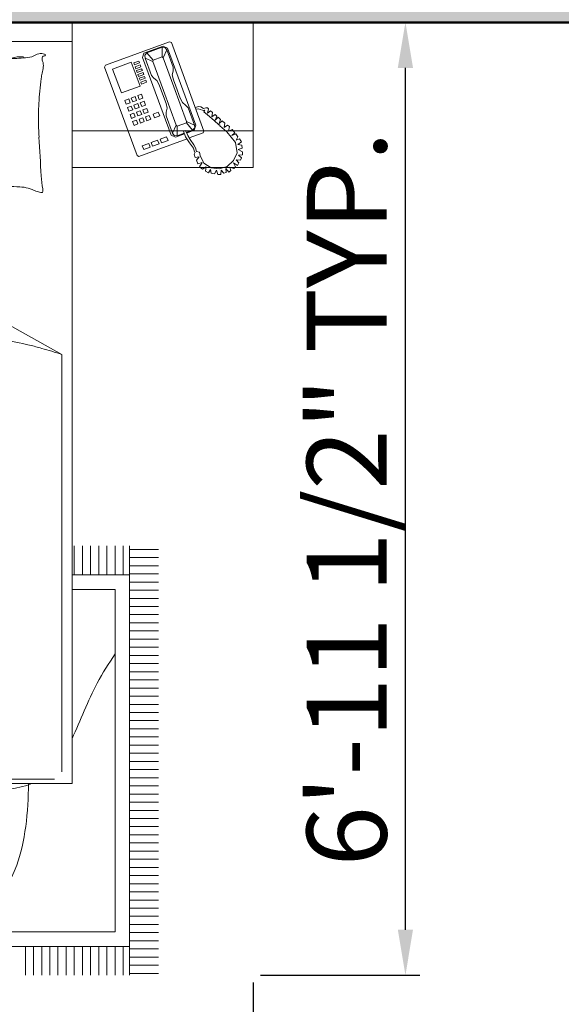
# Model space of a CAD drawing. Units: inches. Extents: x -7 to 1228, y -146 to 1091.
# Tile 12 of 88: x 153 to 200, y 401 to 487. Entities that reach past the tile are written whole.
import ezdxf

# ---------------------------------------------------------------- set-up
doc = ezdxf.new("R2010")
doc.units = ezdxf.units.IN
for name, color, linetype, lineweight in [('A-ANNO-DIMS', 2, 'Continuous', 18), ('A-FURN', 8, 'Continuous', 18), ('A-WALL', 7, 'Continuous', 50), ('A-WALL-PATT', 251, 'Continuous', 13)]:
    doc.layers.add(name, color=color, linetype=linetype, lineweight=lineweight)
doc.styles.add('DIM_FONT', font='SIMPLEX.shx', dxfattribs={"width": 0.8})
doc.styles.get("Standard").update_dxf_attribs({"font": 'arial.ttf'})
doc.dimstyles.new('ISO-25', dxfattribs={"dimtxt": 7, "dimasz": 4, "dimexe": 1.25, "dimexo": 0.625, "dimtad": 1, "dimdec": 1, "dimlunit": 3, "dimtxsty": 'Standard', "dimcen": 2.5, "dimadec": 0, "dimazin": 0, "dimtfac": 1, "dimtdec": 1, "dimtmove": 1, "dimatfit": 3, "dimfxl": 1, "dimarcsym": 0})

# ---------------------------------------------------------------- blocks, each defined once
blk = doc.blocks.new('A$C4F634EDD')
for p, q in [((0.5, 2.6295), (2.3, 2.6295)), ((2.3, 2.6295), (2.3, 0.5295)), ((2.3, 2.6295), (2.8, 2.6295)), ((2.3, 2.2295), (2.3, 2.6295)), ((2.8, 2.6295), (2.8, 2.2295)), ((0.5, 2.5771), (2.3, 2.5771)), ((2.392, 2.5115), (2.5692, 2.5765)), ((2.4985, 2.5445), (2.5516, 2.564)), ((2.5062, 2.5454), (2.5487, 2.561)), ((2.5483, 2.5347), (2.5487, 2.561)), ((2.5487, 2.561), (2.5571, 2.56)), ((2.5516, 2.564), (2.5637, 2.5584)), ((2.5571, 2.56), (2.5615, 2.5536)), ((2.5637, 2.5584), (2.6418, 2.3458)), ((2.5692, 2.5765), (2.574, 2.5743)), ((2.574, 2.5743), (2.6638, 2.3298)), ((2.4946, 2.5331), (2.4985, 2.5445)), ((2.5734, 2.3187), (2.4946, 2.5331)), ((2.5062, 2.5454), (2.5004, 2.5392)), ((2.5004, 2.5392), (2.5013, 2.5315)), ((2.5013, 2.5315), (2.5188, 2.4836)), ((2.5013, 2.5315), (2.5231, 2.5214)), ((2.5235, 2.5256), (2.5062, 2.5454)), ((2.5483, 2.5347), (2.5235, 2.5256)), ((2.5514, 2.5318), (2.5483, 2.5347)), ((2.5615, 2.5536), (2.5514, 2.5318)), ((2.5807, 2.4521), (2.5514, 2.5318)), ((2.5615, 2.5536), (2.5791, 2.5058)), ((2.3898, 2.5066), (2.392, 2.5115)), ((2.4795, 2.2621), (2.3898, 2.5066)), ((2.412, 2.5007), (2.4634, 2.5196)), ((2.4361, 2.4352), (2.412, 2.5007)), ((2.4634, 2.5196), (2.4875, 2.454)), ((2.4842, 2.5232), (2.47, 2.518)), ((2.47, 2.518), (2.472, 2.5127)), ((2.472, 2.5127), (2.4862, 2.5179)), ((2.4881, 2.5126), (2.4739, 2.5074)), ((2.4739, 2.5074), (2.4759, 2.502)), ((2.4759, 2.502), (2.4901, 2.5073)), ((2.492, 2.5019), (2.4778, 2.4967)), ((2.4862, 2.5179), (2.4842, 2.5232)), ((2.4901, 2.5073), (2.4881, 2.5126)), ((2.494, 2.4966), (2.492, 2.5019)), ((2.5231, 2.5214), (2.5235, 2.5256)), ((2.5523, 2.4417), (2.5231, 2.5214)), ((2.5791, 2.5058), (2.5788, 2.4956)), ((2.4778, 2.4967), (2.4798, 2.4914)), ((2.4798, 2.4914), (2.494, 2.4966)), ((2.4959, 2.4913), (2.4817, 2.4861)), ((2.4817, 2.4861), (2.4837, 2.4808)), ((2.4837, 2.4808), (2.4979, 2.486)), ((2.4998, 2.4807), (2.4856, 2.4755)), ((2.4856, 2.4755), (2.4876, 2.4702)), ((2.4876, 2.4702), (2.5018, 2.4754)), ((2.4979, 2.486), (2.4959, 2.4913)), ((2.5018, 2.4754), (2.4998, 2.4807)), ((2.5188, 2.4836), (2.5256, 2.4761)), ((2.5256, 2.4761), (2.5342, 2.4692)), ((2.5788, 2.4956), (2.5767, 2.4848)), ((2.5767, 2.4848), (2.5795, 2.4717)), ((2.4875, 2.454), (2.4361, 2.4352)), ((2.5037, 2.47), (2.4895, 2.4648)), ((2.4895, 2.4648), (2.4915, 2.4595)), ((2.4915, 2.4595), (2.5057, 2.4647)), ((2.5057, 2.4647), (2.5037, 2.47)), ((2.5342, 2.4692), (2.5405, 2.4574)), ((2.5405, 2.4574), (2.547, 2.4397)), ((2.5795, 2.4717), (2.586, 2.454)), ((2.5807, 2.4521), (2.6158, 2.3564)), ((2.5984, 2.4204), (2.586, 2.454)), ((2.4457, 2.4146), (2.4563, 2.4185)), ((2.4563, 2.4185), (2.4602, 2.4078)), ((2.4634, 2.4211), (2.474, 2.425)), ((2.4673, 2.4104), (2.4634, 2.4211)), ((2.474, 2.425), (2.4779, 2.4143)), ((2.4811, 2.4276), (2.4917, 2.4315)), ((2.485, 2.4169), (2.4811, 2.4276)), ((2.4956, 2.4208), (2.485, 2.4169)), ((2.4917, 2.4315), (2.4956, 2.4208)), ((2.5594, 2.4061), (2.547, 2.4397)), ((2.5523, 2.4417), (2.5875, 2.346)), ((2.6047, 2.4086), (2.5984, 2.4204)), ((2.4496, 2.4039), (2.4457, 2.4146)), ((2.4602, 2.4078), (2.4496, 2.4039)), ((2.4528, 2.3951), (2.4635, 2.399)), ((2.4567, 2.3844), (2.4528, 2.3951)), ((2.4635, 2.399), (2.4674, 2.3883)), ((2.4779, 2.4143), (2.4673, 2.4104)), ((2.4706, 2.4016), (2.4812, 2.4055)), ((2.4745, 2.3909), (2.4706, 2.4016)), ((2.4851, 2.3949), (2.4745, 2.3909)), ((2.4812, 2.4055), (2.4851, 2.3949)), ((2.4883, 2.4081), (2.4989, 2.412)), ((2.4922, 2.3975), (2.4883, 2.4081)), ((2.5028, 2.4014), (2.4922, 2.3975)), ((2.4954, 2.3886), (2.5061, 2.3925)), ((2.4989, 2.412), (2.5028, 2.4014)), ((2.5061, 2.3925), (2.51, 2.3819)), ((2.5622, 2.393), (2.5594, 2.4061)), ((2.5601, 2.3822), (2.5622, 2.393)), ((2.6133, 2.4017), (2.6047, 2.4086)), ((2.6201, 2.3941), (2.6133, 2.4017)), ((2.6376, 2.3463), (2.6201, 2.3941)), ((2.6499, 2.3979), (2.6397, 2.3953)), ((2.6551, 2.397), (2.6499, 2.3979)), ((2.6627, 2.392), (2.6551, 2.397)), ((2.6692, 2.394), (2.6627, 2.392)), ((2.6736, 2.3944), (2.6692, 2.394)), ((2.6765, 2.391), (2.6736, 2.3944)), ((2.4674, 2.3883), (2.4567, 2.3844)), ((2.46, 2.3756), (2.4706, 2.3795)), ((2.4639, 2.365), (2.46, 2.3756)), ((2.4745, 2.3689), (2.4639, 2.365)), ((2.4706, 2.3795), (2.4745, 2.3689)), ((2.4777, 2.3821), (2.4883, 2.386)), ((2.4816, 2.3715), (2.4777, 2.3821)), ((2.4922, 2.3754), (2.4816, 2.3715)), ((2.4849, 2.3626), (2.4955, 2.3665)), ((2.4883, 2.386), (2.4922, 2.3754)), ((2.4993, 2.378), (2.4954, 2.3886)), ((2.4955, 2.3665), (2.4994, 2.3559)), ((2.51, 2.3819), (2.4993, 2.378)), ((2.5026, 2.3691), (2.5132, 2.373)), ((2.5065, 2.3585), (2.5026, 2.3691)), ((2.5132, 2.373), (2.5171, 2.3624)), ((2.5238, 2.3769), (2.538, 2.3821)), ((2.5277, 2.3663), (2.5238, 2.3769)), ((2.5419, 2.3715), (2.5277, 2.3663)), ((2.538, 2.3821), (2.5419, 2.3715)), ((2.5598, 2.372), (2.5601, 2.3822)), ((2.5774, 2.3242), (2.5598, 2.372)), ((2.6417, 2.39), (2.6488, 2.391)), ((2.6488, 2.391), (2.6538, 2.3895)), ((2.6538, 2.3895), (2.6596, 2.388)), ((2.6596, 2.388), (2.6626, 2.3867)), ((2.6626, 2.3867), (2.6662, 2.388)), ((2.6662, 2.388), (2.6632, 2.3828)), ((2.6632, 2.3828), (2.6736, 2.3744)), ((2.6736, 2.3744), (2.6922, 2.3593)), ((2.6742, 2.3795), (2.6765, 2.391)), ((2.6824, 2.3858), (2.6742, 2.3795)), ((2.6873, 2.3815), (2.6824, 2.3858)), ((2.6853, 2.369), (2.6873, 2.3815)), ((2.6946, 2.376), (2.6853, 2.369)), ((2.6995, 2.3713), (2.6946, 2.376)), ((2.695, 2.3603), (2.6995, 2.3713)), ((2.7031, 2.3682), (2.695, 2.3603)), ((2.7096, 2.3616), (2.7031, 2.3682)), ((2.4672, 2.3561), (2.4778, 2.36)), ((2.4711, 2.3455), (2.4672, 2.3561)), ((2.4817, 2.3494), (2.4711, 2.3455)), ((2.4778, 2.36), (2.4817, 2.3494)), ((2.4888, 2.352), (2.4849, 2.3626)), ((2.4994, 2.3559), (2.4888, 2.352)), ((2.5171, 2.3624), (2.5065, 2.3585)), ((2.5774, 2.3242), (2.5875, 2.346)), ((2.5875, 2.346), (2.5905, 2.3431)), ((2.5905, 2.3431), (2.5901, 2.3168)), ((2.6154, 2.3522), (2.5905, 2.3431)), ((2.6158, 2.3564), (2.6154, 2.3522)), ((2.6154, 2.3522), (2.6327, 2.3324)), ((2.6376, 2.3463), (2.6158, 2.3564)), ((2.6327, 2.3324), (2.6385, 2.3386)), ((2.6418, 2.3458), (2.6369, 2.332)), ((2.6385, 2.3386), (2.6376, 2.3463)), ((2.6922, 2.3593), (2.7051, 2.3473)), ((2.7051, 2.3473), (2.7079, 2.3475)), ((2.7062, 2.351), (2.7096, 2.3616)), ((2.7147, 2.3578), (2.7062, 2.351)), ((2.7079, 2.3475), (2.7079, 2.3443)), ((2.7079, 2.3443), (2.727, 2.3277)), ((2.7214, 2.3517), (2.7147, 2.3578)), ((2.7196, 2.34), (2.7214, 2.3517)), ((2.7286, 2.3466), (2.7196, 2.34)), ((2.7346, 2.3423), (2.7286, 2.3466)), ((2.732, 2.3295), (2.7346, 2.3423)), ((2.8, 2.3301), (2.3, 2.3301)), ((2.561, 2.3141), (2.5433, 2.3076)), ((2.5649, 2.3035), (2.561, 2.3141)), ((2.5855, 2.3131), (2.5734, 2.3187)), ((2.5818, 2.3178), (2.5774, 2.3242)), ((2.5901, 2.3168), (2.5818, 2.3178)), ((2.6104, 2.3222), (2.5855, 2.3131)), ((2.5901, 2.3168), (2.6097, 2.324)), ((2.613, 2.3312), (2.6077, 2.3293)), ((2.6077, 2.3293), (2.6135, 2.3141)), ((2.6192, 2.3174), (2.613, 2.3312)), ((2.6135, 2.3141), (2.6244, 2.2977)), ((2.6153, 2.3261), (2.6327, 2.3324)), ((2.6369, 2.332), (2.6161, 2.3243)), ((2.626, 2.3069), (2.6192, 2.3174)), ((2.6616, 2.3249), (2.6234, 2.3109)), ((2.6638, 2.3298), (2.6616, 2.3249)), ((2.727, 2.3277), (2.7512, 2.2983)), ((2.7423, 2.3345), (2.732, 2.3295)), ((2.7406, 2.3172), (2.7495, 2.325)), ((2.7519, 2.3218), (2.7406, 2.3172)), ((2.7495, 2.325), (2.7423, 2.3345)), ((2.7575, 2.3144), (2.7519, 2.3218)), ((2.7526, 2.3045), (2.7575, 2.3144)), ((2.6172, 2.3086), (2.4844, 2.2599)), ((2.5114, 2.2959), (2.4936, 2.2894)), ((2.4936, 2.2894), (2.4976, 2.2788)), ((2.4976, 2.2788), (2.5153, 2.2853)), ((2.5153, 2.2853), (2.5114, 2.2959)), ((2.5362, 2.305), (2.5185, 2.2985)), ((2.5185, 2.2985), (2.5224, 2.2879)), ((2.5224, 2.2879), (2.5401, 2.2944)), ((2.5401, 2.2944), (2.5362, 2.305)), ((2.5433, 2.3076), (2.5472, 2.297)), ((2.5472, 2.297), (2.5649, 2.3035)), ((2.6244, 2.2977), (2.6349, 2.2825)), ((2.6365, 2.2916), (2.626, 2.3069)), ((2.6349, 2.2825), (2.638, 2.273)), ((2.6407, 2.2834), (2.6365, 2.2916)), ((2.6438, 2.2739), (2.6407, 2.2834)), ((2.7512, 2.2983), (2.756, 2.2695)), ((2.7622, 2.308), (2.7526, 2.3045)), ((2.7574, 2.2924), (2.7673, 2.2997)), ((2.7687, 2.2905), (2.7574, 2.2924)), ((2.7587, 2.279), (2.7699, 2.2828)), ((2.7673, 2.2997), (2.7622, 2.308)), ((2.7699, 2.2828), (2.7687, 2.2905)), ((2.4844, 2.2599), (2.4795, 2.2621)), ((2.6399, 2.2712), (2.6374, 2.2659)), ((2.6374, 2.2659), (2.6398, 2.257)), ((2.638, 2.273), (2.6399, 2.2712)), ((2.6398, 2.257), (2.6509, 2.259)), ((2.6509, 2.259), (2.6431, 2.2492)), ((2.6519, 2.2716), (2.6438, 2.2739)), ((2.6535, 2.2628), (2.6519, 2.2716)), ((2.6636, 2.2409), (2.6535, 2.2628)), ((2.756, 2.2695), (2.7459, 2.2483)), ((2.7708, 2.2725), (2.7587, 2.279)), ((2.759, 2.2637), (2.7706, 2.2643)), ((2.7676, 2.2559), (2.759, 2.2637)), ((2.7645, 2.2498), (2.7676, 2.2559)), ((2.7706, 2.2643), (2.7708, 2.2725)), ((2.8, 2.2295), (2.3, 2.2295)), ((2.6431, 2.2492), (2.6473, 2.2398)), ((2.6473, 2.2398), (2.6592, 2.2429)), ((2.6592, 2.2429), (2.6521, 2.2314)), ((2.6521, 2.2314), (2.6598, 2.2248)), ((2.6598, 2.2248), (2.6697, 2.2309)), ((2.6836, 2.2287), (2.6636, 2.2409)), ((2.6697, 2.2309), (2.6684, 2.219)), ((2.7063, 2.2256), (2.6836, 2.2287)), ((2.7284, 2.2317), (2.7063, 2.2256)), ((2.7459, 2.2483), (2.7284, 2.2317)), ((2.7386, 2.2208), (2.7354, 2.2306)), ((2.7354, 2.2306), (2.7462, 2.2264)), ((2.7509, 2.2314), (2.7459, 2.2418)), ((2.7459, 2.2418), (2.7568, 2.2352)), ((2.7462, 2.2264), (2.7509, 2.2314)), ((2.7529, 2.2505), (2.7645, 2.2498)), ((2.7607, 2.2424), (2.7529, 2.2505)), ((2.7568, 2.2352), (2.7607, 2.2424)), ((2.6684, 2.219), (2.6761, 2.2145)), ((2.6761, 2.2145), (2.6821, 2.2237)), ((2.6821, 2.2237), (2.6843, 2.2135)), ((2.6843, 2.2135), (2.6927, 2.2117)), ((2.6927, 2.2117), (2.6986, 2.222)), ((2.6986, 2.222), (2.7019, 2.2098)), ((2.7019, 2.2098), (2.7102, 2.2104)), ((2.7102, 2.2104), (2.7113, 2.2218)), ((2.7113, 2.2218), (2.7192, 2.2137)), ((2.7192, 2.2137), (2.7255, 2.2152)), ((2.7255, 2.2152), (2.7242, 2.2265)), ((2.7242, 2.2265), (2.7324, 2.2165)), ((2.7324, 2.2165), (2.7386, 2.2208)), ((1.5035, 2.141), (2.2716, 1.7136)), ((2.2716, 0.5617), (2.2716, 1.7136)), ((2.3061, 1.1052), (2.3061, 1.1852)), ((2.3286, 1.1052), (2.3286, 1.1852)), ((2.3511, 1.1052), (2.3511, 1.1852)), ((2.3736, 1.1052), (2.3736, 1.1852)), ((2.3961, 1.1052), (2.3961, 1.1852)), ((2.4186, 1.1052), (2.4186, 1.1852)), ((2.4411, 1.1052), (2.4411, 1.1852)), ((2.4588, 1.1852), (2.4588, 0)), ((2.4588, 1.1753), (2.5388, 1.1753)), ((2.4588, 1.1528), (2.5388, 1.1528)), ((2.4588, 1.1303), (2.5388, 1.1303)), ((2.3, 1.1052), (2.4588, 1.1052)), ((2.4588, 1.1078), (2.5388, 1.1078)), ((2.3, 1.0652), (2.4188, 1.0652)), ((2.4188, 1.0652), (2.4188, 0.12)), ((2.4588, 1.0853), (2.5388, 1.0853)), ((2.4588, 1.0628), (2.5388, 1.0628)), ((2.4588, 1.0403), (2.5388, 1.0403)), ((2.4588, 1.0178), (2.5388, 1.0178)), ((2.4588, 0.9953), (2.5388, 0.9953)), ((2.4588, 0.9728), (2.5388, 0.9728)), ((2.4588, 0.9503), (2.5388, 0.9503)), ((2.4588, 0.9278), (2.5388, 0.9278)), ((2.4588, 0.9053), (2.5388, 0.9053)), ((2.4588, 0.8828), (2.5388, 0.8828)), ((2.4588, 0.8603), (2.5388, 0.8603)), ((2.4588, 0.8378), (2.5388, 0.8378)), ((2.4588, 0.8153), (2.5388, 0.8153)), ((2.4588, 0.7928), (2.5388, 0.7928)), ((2.4588, 0.7703), (2.5388, 0.7703)), ((2.4588, 0.7478), (2.5388, 0.7478)), ((2.4588, 0.7253), (2.5388, 0.7253)), ((2.4588, 0.7028), (2.5388, 0.7028)), ((2.4588, 0.6803), (2.5388, 0.6803)), ((2.4588, 0.6578), (2.5388, 0.6578)), ((2.4588, 0.6353), (2.5388, 0.6353)), ((2.4588, 0.6128), (2.5388, 0.6128)), ((2.4588, 0.5903), (2.5388, 0.5903)), ((2.4588, 0.5678), (2.5388, 0.5678)), ((2.4588, 0.5453), (2.5388, 0.5453)), ((2.3, 0.5295), (0.5, 0.5295)), ((0.5458, 0.5417), (2.2516, 0.5417)), ((2.4588, 0.5228), (2.5388, 0.5228)), ((2.4588, 0.5003), (2.5388, 0.5003)), ((2.4588, 0.4778), (2.5388, 0.4778)), ((2.4588, 0.4553), (2.5388, 0.4553)), ((2.4588, 0.4328), (2.5388, 0.4328)), ((2.4588, 0.4103), (2.5388, 0.4103)), ((2.4588, 0.3878), (2.5388, 0.3878)), ((2.4588, 0.3653), (2.5388, 0.3653)), ((2.4588, 0.3428), (2.5388, 0.3428)), ((2.4588, 0.3203), (2.5388, 0.3203)), ((2.4588, 0.2978), (2.5388, 0.2978)), ((2.4588, 0.2753), (2.5388, 0.2753)), ((2.4588, 0.2528), (2.5388, 0.2528)), ((2.4588, 0.2303), (2.5388, 0.2303)), ((2.4588, 0.2078), (2.5388, 0.2078)), ((2.4588, 0.1853), (2.5388, 0.1853)), ((2.4588, 0.1628), (2.5388, 0.1628)), ((2.4588, 0.1403), (2.5388, 0.1403)), ((2.4188, 0.12), (0.3786, 0.12)), ((2.4588, 0.1178), (2.5388, 0.1178)), ((2.4588, 0.0953), (2.5388, 0.0953)), ((2.4588, 0.08), (0.3386, 0.08)), ((2.1711, 0), (2.1711, 0.08)), ((2.1936, 0), (2.1936, 0.08)), ((2.2161, 0), (2.2161, 0.08)), ((2.2386, 0), (2.2386, 0.08)), ((2.2611, 0), (2.2611, 0.08)), ((2.2836, 0), (2.2836, 0.08)), ((2.3061, 0), (2.3061, 0.08)), ((2.3286, 0), (2.3286, 0.08)), ((2.3511, 0), (2.3511, 0.08)), ((2.3736, 0), (2.3736, 0.08)), ((2.3961, 0), (2.3961, 0.08)), ((2.4186, 0), (2.4186, 0.08)), ((2.4411, 0), (2.4411, 0.08)), ((2.4588, 0.0728), (2.5388, 0.0728)), ((2.4588, 0.0503), (2.5388, 0.0503)), ((2.4588, 0.0278), (2.5388, 0.0278)), ((2.4588, 0.0053), (2.5388, 0.0053))]:
    blk.add_line(p, q)
for centre, radius, start, end in [((2.1021, 3.3501), 0.8208, 271.9079, 275.2592), ((2.1588, 2.4357), 0.0992, 85.7841, 105.9352), ((2.1724, 2.5864), 0.0539, 275.2592, 300.6513), ((2.2146, 2.5152), 0.0289, 85.6975, 120.6513), ((2.2149, 2.519), 0.0251, 68.2117, 85.6975), ((2.2331, 2.5288), 0.0156, 158.0096, 201.421), ((2.2226, 2.533), 0.00428, 78.1069, 158.0096), ((2.224, 2.5395), 0.00232, 258.1069, 19.564), ((2.2229, 2.5391), 0.00342, 19.564, 68.2117), ((1.977, 2.5413), 0.246, 347.8905, 351.8665), ((2.1881, 2.5111), 0.0328, 351.8665, 21.421), ((3.1198, 2.3525), 0.9131, 172.3191, 176.6313), ((2.4114, 2.448), 0.1983, 167.8905, 172.3191), ((2.8858, 2.3663), 0.6787, 176.6313, 181.6331), ((3.5721, 2.3859), 1.3652, 181.6331, 183.055), ((15.8249, 3.0398), 13.6356, 183.05496, 183.50486), ((2.5355, 2.2258), 0.3212, 183.5049, 189.9984), ((2.0833, 1.0141), 1.164, 86.426, 89.7135), ((2.1467, 2.0302), 0.1459, 77.131, 86.426), ((2.1691, 2.1283), 0.0453, 62.7159, 77.131), ((2.2251, 2.2367), 0.0767, 242.7159, 253.7788), ((2.2281, 2.247), 0.0875, 253.7788, 262.8796), ((2.2174, 2.1615), 0.00132, 262.8796, 343.3022), ((2.2001, 2.1667), 0.0193, 343.3022, 9.9984), ((1.2737, -2.2227), 4.0646, 77.0745, 79.2724), ((2.0359, 1.0981), 0.6574, 74.0648, 77.0745), ((1.7125, -0.0344), 1.8351, 72.2636, 74.0648)]:
    blk.add_arc(centre, radius, start, end)
for points, knots in [([(2.3, 0.6535), (2.3236, 0.7026), (2.3554, 0.7914), (2.4015, 0.8608), (2.4188, 0.8868)], [1893.525221, 1893.525221, 1893.525221, 1893.525221, 2051.902476, 2146.74457, 2146.74457, 2146.74457, 2146.74457]), ([(2.1796, 0.5295), (2.1798, 0.4519), (2.1548, 0.2369), (2.0487, 0.164), (1.9846, 0.12)], [2202.034493, 2202.034493, 2202.034493, 2202.034493, 2357.807635, 2594.446174, 2594.446174, 2594.446174, 2594.446174])]:
    blk.add_open_spline(points, degree=3, knots=knots)
blk.add_open_spline([(1.9003, 0.5295), (2.0065, 0.514), (2.1132, 0.4978), (2.1894, 0.5295)], degree=3)
at = {"style": 'DIM_FONT', "width": 0.8, "flags": 9}
for tag, p in [('YSIZE', (0.5, 2.6295)), ('XSIZE', (0.5, 2.6295)), ('XSIZE', (2.2985, 2.6295)), ('YSIZE', (2.2985, 2.6295))]:
    blk.add_attdef(tag, p, '', height=0.0005, dxfattribs=at)
blk = doc.blocks.new('*D24')
at = {"layer": 'A-ANNO-DIMS', "color": 0, "lineweight": -2, "transparency": 16777216}
for p, q in [((84.435, 402.798), (84.435, 388.824)), ((173.431, 402.798), (173.431, 388.824)), ((88.435, 390.074), (169.431, 390.074))]:
    blk.add_line(p, q, dxfattribs=at)
at = {"layer": 'A-ANNO-DIMS', "color": 0, "transparency": 16777216}
for points in [[(88.435, 390.741), (88.435, 389.407), (84.435, 390.074)], [(169.431, 390.741), (169.431, 389.407), (173.431, 390.074)]]:
    blk.add_solid(points, dxfattribs=at)
at = {"layer": 'Defpoints', "color": 0, "transparency": 16777216}
for p in [(84.435, 403.423), (173.431, 403.423), (173.431, 390.074)]:
    blk.add_point(p, dxfattribs=at)
at = {"layer": 'A-ANNO-DIMS', "color": 0, "transparency": 16777216, "insert": (128.933, 394.259), "char_height": 7, "attachment_point": 5}
blk.add_mtext('BED 7\'-5" TYP.', dxfattribs=at)
blk = doc.blocks.new('*D25')
at = {"layer": 'A-ANNO-DIMS', "color": 0, "lineweight": -2, "transparency": 16777216}
for p, q in [((174.056, 487.016), (188.031, 487.016)), ((186.781, 407.423), (186.781, 483.016)), ((174.056, 403.423), (188.031, 403.423))]:
    blk.add_line(p, q, dxfattribs=at)
at = {"layer": 'A-ANNO-DIMS', "color": 0, "transparency": 16777216}
for points in [[(186.114, 483.016), (187.447, 483.016), (186.781, 487.016)], [(186.114, 407.423), (187.447, 407.423), (186.781, 403.423)]]:
    blk.add_solid(points, dxfattribs=at)
at = {"layer": 'Defpoints', "color": 0, "transparency": 16777216}
for p in [(173.431, 487.016), (186.781, 487.016), (173.431, 403.423)]:
    blk.add_point(p, dxfattribs=at)
at = {"layer": 'A-ANNO-DIMS', "color": 0, "transparency": 16777216, "insert": (182.536, 445.22), "char_height": 7, "attachment_point": 5, "rotation": 90}
blk.add_mtext('6\'-11 1/2" TYP.', dxfattribs=at)

msp = doc.modelspace()

# ---------------------------------------------------------------- hatches: boundary and pattern name
at = {"layer": 'A-WALL-PATT'}
h = msp.add_hatch(color=256, dxfattribs=at)
h.dxf.hatch_style = 1
h.paths.add_polyline_path([(69, 568), (60, 568), (60, 493), (63.289, 493), (69, 493)])
h.paths.add_polyline_path([(69, 662.405), (60, 662.405), (60, 586), (69, 586)], flags=17)
h.paths.add_polyline_path([(69, 723), (184, 723), (184, 734), (179, 734), (179, 728), (69, 728), (69, 741.623), (60, 741.623), (60, 698.405), (69, 698.405)], flags=17)
h.paths.add_polyline_path([(69, 782), (231, 782), (231, 728), (231, 723), (231, 586), (236, 586), (236, 787), (69, 787), (69, 800.126), (60, 800.126), (60, 765.623), (69, 765.623)])
h.paths.add_polyline_path([(184, 842), (189, 842), (189, 848), (173, 848), (173, 842), (179, 842), (179, 787), (184, 787)])
h.paths.add_polyline_path([(118.22, 69), (69, 69), (69, 60), (118.22, 60)])
h.paths.add_polyline_path([(227, 69), (154.22, 69), (154.22, 60), (227, 60)])
h.paths.add_polyline_path([(236, 60), (232.711, 60), (227, 60), (227, 36), (236, 36)])
h.paths.add_polyline_path([(389, 60), (380, 60), (380, 36), (389, 36)])
h.paths.add_polyline_path([(384, 181), (380, 181), (380, 115), (380, 78), (384, 78)])
h.paths.add_polyline_path([(380, 115), (334.547, 115), (334.547, 109), (380, 109)])
h.paths.add_polyline_path([(274.547, 115), (236, 115), (236, 201), (232.711, 201), (231, 201), (231, 78), (236, 78), (236, 109), (274.547, 109)])
h.paths.add_polyline_path([(69, 123), (60, 123), (60, 78), (69, 78)])
h.paths.add_polyline_path([(69, 201), (60, 201), (60, 159), (69, 159)])
h.paths.add_polyline_path([(143, 219), (69, 219), (69, 213), (143, 213)], flags=17)
h.paths.add_polyline_path([(189, 219), (184, 219), (184, 274), (231, 274), (231, 219), (236, 219), (236, 279), (184, 279), (184, 297), (179, 297), (179, 279), (69, 279), (69, 290.912), (60, 290.912), (60, 262.179), (69, 262.179), (69, 274), (179, 274), (179, 219), (173, 219), (173, 213), (189, 213)])
h.paths.add_polyline_path([(69, 238.179), (60, 238.179), (60, 219), (69, 219)], flags=17)
h.paths.add_polyline_path([(69, 333), (60, 333), (60, 314.912), (69, 314.912), (69, 316.965)])
h.paths.add_polyline_path([(190, 338), (184, 338), (69, 338), (69, 333), (179, 333), (179, 327), (184, 327), (184, 333.021), (190, 333.046)])
h.paths.add_polyline_path([(69, 386.806), (60, 386.806), (60, 351), (69, 351)])
h.paths.add_polyline_path([(69, 475), (60, 475), (60, 422.806), (69, 422.806)])
h.paths.add_polyline_path([(236, 475), (231, 475), (231, 351.238), (236, 351.238)])
h.paths.add_polyline_path([(384, 475), (380, 475), (380, 362), (384, 362)])
h.paths.add_polyline_path([(547, 307), (439, 307), (439, 356), (445, 356), (445, 362), (433, 362), (433, 307), (380, 307), (380, 244), (380, 241), (384, 241), (384, 301), (433, 301), (433, 277), (439, 277), (439, 301), (547, 301)])
h.paths.add_polyline_path([(547, 241), (439, 241), (439, 247), (433, 247), (433, 235), (547, 235)])
h.paths.add_polyline_path([(450, 69), (440.286, 69), (424.889, 69), (389, 69), (389, 60), (450, 60)])
h.paths.add_polyline_path([(547, 69), (486, 69), (486, 60), (547, 60)])
h.paths.add_polyline_path([(556, 148.268), (547, 148.268), (547, 78), (556, 78)])
h.paths.add_polyline_path([(556, 223), (547, 223), (547, 195), (547, 184.268), (556, 184.268)])
h.paths.add_polyline_path([(556, 311.192), (547, 311.192), (547, 273.075), (556, 273.075)])
h.paths.add_polyline_path([(556, 344), (552.711, 344), (547, 344), (547, 335.192), (556, 335.192)])
h.paths.add_polyline_path([(556, 249.075), (547, 249.075), (547, 241), (556, 241)])
h.paths.add_polyline_path([(547, 362), (475, 362), (475, 356), (547, 356)], flags=0)
h.paths.add_polyline_path([(556, 399.621), (547, 399.621), (547, 362), (556, 362)])
h.paths.add_polyline_path([(556, 475), (547, 475), (547, 435.621), (556, 435.621)])
h.paths.add_polyline_path([(547, 493), (389, 493), (389, 487), (547, 487)])
h.paths.add_polyline_path([(380, 493), (278, 493), (278, 487), (380, 487)])
h.paths.add_polyline_path([(227, 493), (69, 493), (69, 487), (227, 487)])
h.paths.add_polyline_path([(643, 122.445), (634, 122.445), (634, 78), (643, 78)])
h.paths.add_polyline_path([(702.5, 69), (692.786, 69), (677.389, 69), (643, 69), (643, 60), (702.5, 60)])
h.paths.add_polyline_path([(798, 69), (738.5, 69), (738.5, 60), (798, 60)])
h.paths.add_polyline_path([(807, 60), (803.711, 60), (798, 60), (798, 36), (807, 36)])
h.paths.add_polyline_path([(807, 109), (846.751, 109), (846.751, 115), (807, 115), (807, 159), (802, 159), (802, 78), (807, 78)])
h.paths.add_polyline_path([(807, 201), (802, 201), (802, 195), (807, 195)])
h.paths.add_polyline_path([(643, 201), (634, 201), (634, 158.445), (643, 158.445)])
h.paths.add_polyline_path([(756, 225), (751, 225), (751, 219), (643, 219), (643, 213), (756, 213)])
h.paths.add_polyline_path([(643, 240.848), (634, 240.848), (634, 219), (643, 219)])
h.paths.add_polyline_path([(643, 274), (643, 288.629), (634, 288.629), (634, 264.848), (643, 264.848)])
h.paths.add_polyline_path([(802, 279), (756, 279), (756, 297), (751, 297), (751, 279), (643, 279), (643, 274), (751, 274), (751, 255), (756, 255), (756, 274), (802, 274)])
h.paths.add_polyline_path([(807, 333), (803.711, 333), (802, 333), (802, 279), (802, 274), (802, 219), (807, 219)])
h.paths.add_polyline_path([(956, 182), (951, 182), (951, 115), (906.751, 115), (906.751, 109), (951, 109), (951, 78), (956, 78)])
h.paths.add_polyline_path([(960, 60), (951, 60), (951, 36), (960, 36)])
h.paths.add_polyline_path([(1021, 69), (1005.781, 69), (960, 69), (960, 60), (1021, 60)])
h.paths.add_polyline_path([(956, 224), (951, 224), (951, 218), (956, 218)])
h.paths.add_polyline_path([(956, 302), (1004, 302), (1004, 278), (1010, 278), (1010, 302), (1118, 302), (1118, 290.809), (1127, 290.809), (1127, 326.968), (1118, 326.968), (1118, 320.966), (1118, 307), (1010, 307), (1010, 356), (1016, 356), (1016, 362), (1004, 362), (1004, 307), (951, 307), (951, 244), (951, 242), (954.289, 242), (956, 242)])
h.paths.add_polyline_path([(643, 333), (634, 333), (634, 312.629), (643, 312.629), (643, 316.965)])
h.paths.add_polyline_path([(756, 338), (643, 338), (643, 333), (751, 333), (751, 327), (756, 327)])
h.paths.add_polyline_path([(643, 388), (634, 388), (634, 351), (643, 351)])
h.paths.add_polyline_path([(807, 357), (802, 357), (802, 351), (807, 351)])
h.paths.add_polyline_path([(807, 475), (802, 475), (802, 393), (807, 393)])
h.paths.add_polyline_path([(643, 475), (634, 475), (634, 424), (643, 424)])
h.paths.add_polyline_path([(798, 493), (643, 493), (643, 487), (798, 487)])
h.paths.add_polyline_path([(634, 493), (556, 493), (556, 487), (634, 487)])
h.paths.add_polyline_path([(813, 493), (807, 493), (807, 487), (813, 487)])
h.paths.add_polyline_path([(951, 493), (849, 493), (849, 487), (951, 487)])
h.paths.add_polyline_path([(956, 484), (951, 484), (951, 374), (956, 374)])
h.paths.add_polyline_path([(1109, 493), (969, 493), (969, 487), (1109, 487)])
h.paths.add_polyline_path([(1127, 484), (1118, 484), (1118, 450.641), (1127, 450.641)])
h.paths.add_polyline_path([(1127, 414.641), (1118, 414.641), (1118, 365), (1127, 365)])
h.paths.add_polyline_path([(1109, 362), (1046, 362), (1046, 356), (1109, 356)], flags=17)
h.paths.add_polyline_path([(1127, 356), (1123.454, 356), (1118, 356), (1118, 350.968), (1127, 350.968)], flags=0)
h.paths.add_polyline_path([(1127, 266.809), (1118, 266.809), (1118, 262.361), (1118, 242), (1127, 242)], flags=17)
h.paths.add_polyline_path([(1118, 242), (1010, 242), (1010, 248), (1004, 248), (1004, 237), (1118, 237)])
h.paths.add_polyline_path([(1127, 224), (1118, 224), (1118, 170), (1127, 170)])
h.paths.add_polyline_path([(1127, 134), (1118, 134), (1118, 78), (1127, 78)])
h.paths.add_polyline_path([(1118, 69), (1057, 69), (1057, 60), (1118, 60)])
h.paths.add_polyline_path([(227, 571.546), (227, 574), (69, 574), (69, 568), (227, 568)])
h.paths.add_polyline_path([(380, 571.546), (380, 574), (278, 574), (278, 568), (380, 568)])
h.paths.add_polyline_path([(242, 574), (236, 574), (236, 568), (242, 568)])
h.paths.add_polyline_path([(547, 571.546), (547, 574), (389, 574), (389, 568), (547, 568)])
h.paths.add_polyline_path([(384, 733), (380, 733), (380, 586), (384, 586)])
h.paths.add_polyline_path([(556, 646), (634, 646), (634, 655), (547, 655), (547, 586), (556, 586)])
h.paths.add_polyline_path([(634, 574), (556, 574), (556, 568), (634, 568)])
h.paths.add_polyline_path([(643, 655), (634, 655), (634, 586), (643, 586)])
h.paths.add_polyline_path([(798, 574), (643, 574), (643, 568), (798, 568)])
h.paths.add_polyline_path([(643, 663.854), (634, 663.854), (634, 655), (643, 655)])
h.paths.add_polyline_path([(556, 676.967), (547, 676.967), (547, 655), (556, 655)])
h.paths.add_polyline_path([(556, 733), (547, 733), (547, 712.967), (556, 712.967)])
h.paths.add_polyline_path([(643, 710), (634, 710), (634, 699.854), (643, 699.854)])
h.paths.add_polyline_path([(807, 668), (802, 668), (802, 586), (807, 586)])
h.paths.add_polyline_path([(951, 574), (849, 574), (849, 568), (951, 568)])
h.paths.add_polyline_path([(956, 691), (951, 691), (951, 577), (956, 577)])
h.paths.add_polyline_path([(1109, 574), (969, 574), (969, 568), (1109, 568)])
h.paths.add_polyline_path([(1127, 643.403), (1118, 643.403), (1118, 577), (1127, 577)])
h.paths.add_polyline_path([(1127, 568), (1123.454, 568), (1118, 568), (1118, 493), (1127, 493)])
h.paths.add_polyline_path([(1127, 733), (1118, 733), (1118, 679.403), (1127, 679.403)])
h.paths.add_polyline_path([(1127, 777.348), (1118, 777.348), (1118, 770.035), (1118, 751), (1127, 751)], flags=17)
h.paths.add_polyline_path([(1118, 751), (1010, 751), (1010, 757), (1004, 757), (1004, 745), (1118, 745)])
h.paths.add_polyline_path([(956, 811), (1004, 811), (1004, 787), (1010, 787), (1010, 811), (1017.874, 811), (1017.874, 811.627, -0.414214), (1018.247, 812), (1031.978, 812, -0.414214), (1032.351, 811.627), (1032.351, 811), (1118, 811), (1118, 801.348), (1127, 801.348), (1127, 834.685), (1118, 834.685), (1118, 830.238), (1118, 817), (1010, 817), (1010, 866), (1016, 866), (1016, 872), (1004, 872), (1004, 817), (956, 817), (956, 866), (951, 866), (951, 751), (954.289, 751), (956, 751)])
h.paths.add_polyline_path([(1118, 872), (1046, 872), (1046, 866), (1118, 866)], flags=17)
h.paths.add_polyline_path([(1127, 924.711), (1118, 924.711), (1118, 884), (1127, 884)])
h.paths.add_polyline_path([(1127, 866), (1123.711, 866), (1118, 866), (1118, 858.685), (1127, 858.685)], flags=17)
h.paths.add_polyline_path([(956, 983), (951, 983), (951, 952), (807, 952), (807, 983), (802, 983), (802, 902), (807, 902), (807, 946), (951, 946), (951, 884), (956, 884)])
h.paths.add_polyline_path([(807, 842), (802, 842), (802, 787), (756, 787), (756, 806), (751, 806), (751, 787), (643, 787), (643, 782), (751, 782), (751, 764), (756, 764), (756, 782), (802, 782), (802, 728), (807, 728)])
h.paths.add_polyline_path([(756, 848), (643, 848), (643, 842), (751, 842), (751, 836), (756, 836)])
h.paths.add_polyline_path([(756, 734), (751, 734), (751, 728), (643, 728), (643, 723), (756, 723)])
h.paths.add_polyline_path([(643, 749.791), (634, 749.791), (634, 728), (637.289, 728), (643, 728)])
h.paths.add_polyline_path([(643, 805.405), (634, 805.405), (634, 773.791), (643, 773.791)])
h.paths.add_polyline_path([(643, 896.663), (634, 896.663), (634, 860), (637.289, 860), (643, 860)])
h.paths.add_polyline_path([(643, 842), (634, 842), (634, 829.405), (643, 829.405)])
h.paths.add_polyline_path([(643, 983), (634, 983), (634, 932.663), (643, 932.663)])
h.paths.add_polyline_path([(1127, 983), (1118, 983), (1118, 960.711), (1127, 960.711)])
h.paths.add_polyline_path([(1118, 1001), (1077.525, 1001), (1077.525, 992), (1118, 992)])
h.paths.add_polyline_path([(1041.525, 1001), (960, 1001), (960, 992), (1041.525, 992)])
h.paths.add_polyline_path([(960, 1025), (951, 1025), (951, 1001), (954.289, 1001), (960, 1001)])
h.paths.add_polyline_path([(807, 1025), (798, 1025), (798, 1001), (807, 1001)])
h.paths.add_polyline_path([(798, 1001), (738.5, 1001), (738.5, 992), (798, 992)])
h.paths.add_polyline_path([(702.5, 1001), (643, 1001), (643, 992), (702.5, 992)])
h.paths.add_polyline_path([(547, 1001), (499.113, 1001), (499.113, 992), (547, 992)])
h.paths.add_polyline_path([(463.113, 1001), (389, 1001), (389, 992), (463.113, 992)])
h.paths.add_polyline_path([(389, 1025), (380, 1025), (380, 1022), (380, 1001), (383.289, 1001), (389, 1001)])
h.paths.add_polyline_path([(236, 1025), (227, 1025), (227, 1001), (236, 1001)])
h.paths.add_polyline_path([(236, 983), (231, 983), (231, 860), (236, 860)])
h.paths.add_polyline_path([(274.547, 952), (236, 952), (236, 946), (274.547, 946)])
h.paths.add_polyline_path([(380, 952), (334.547, 952), (334.547, 946), (380, 946)])
h.paths.add_polyline_path([(384, 983), (380, 983), (380, 884), (383.289, 884), (384, 884)])
h.paths.add_polyline_path([(227, 1001), (155.012, 1001), (155.012, 992), (162.875, 992), (227, 992)])
h.paths.add_polyline_path([(119.012, 1001), (69, 1001), (69, 992), (119.012, 992)])
h.paths.add_polyline_path([(69, 983), (60, 983), (60, 922.987), (69, 922.987)])
h.paths.add_polyline_path([(69, 886.987), (60, 886.987), (60, 860), (63.289, 860), (69, 860)])
h.paths.add_polyline_path([(143, 848), (69, 848), (69, 842), (143, 842)])

# ---------------------------------------------------------------- linework, layer by layer
at = {"layer": 'A-WALL'}
msp.add_line((231, 487), (69, 487), dxfattribs=at)

# ---------------------------------------------------------------- block references
at = {"layer": 'A-FURN', "xscale": 31.78426361944092, "yscale": 31.78426361944092, "zscale": 31.78426361944092}
msp.add_blockref('A$C4F634EDD', (84.435, 403.423), dxfattribs=at)

# ---------------------------------------------------------------- dimensions: what is measured, and where the dimension line sits
at = {"layer": 'A-ANNO-DIMS'}
dim = msp.add_linear_dim(base=(186.781, 487.016), p1=(173.431, 403.423), p2=(173.431, 487.016), angle=90, text='<> TYP.', dimstyle='ISO-25', override={"dimdec": 1, "dimlfac": 1, "dimrnd": 0, "dimzin": 1, "dimdsep": 46, "dimlunit": 4, "dimfrac": 2}, dxfattribs=at)
dim.commit()
dim.dimension.update_dxf_attribs({"geometry": '*D25', "text_midpoint": (182.536, 445.22)})
dim = msp.add_linear_dim(base=(173.431, 390.074), p1=(84.435, 403.423), p2=(173.431, 403.423), text='BED <> TYP.', dimstyle='ISO-25', override={"dimdec": 1, "dimlfac": 1, "dimrnd": 0, "dimzin": 1, "dimdsep": 46, "dimlunit": 4, "dimfrac": 2}, dxfattribs=at)
dim.commit()
dim.dimension.update_dxf_attribs({"geometry": '*D24', "text_midpoint": (128.933, 394.259)})

doc.saveas('drawing.dxf')
